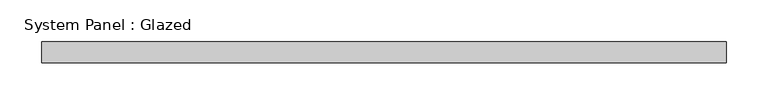
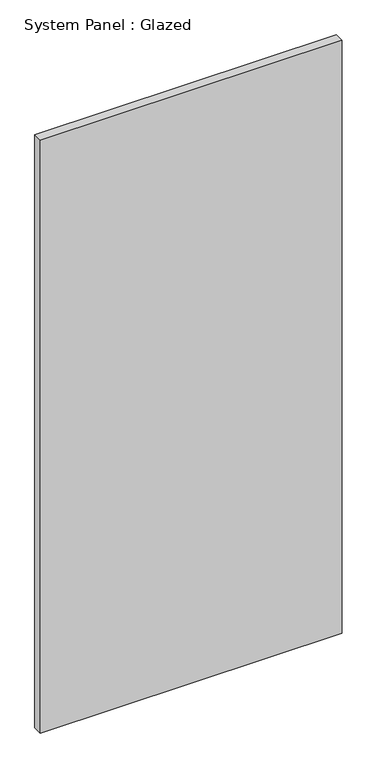
"""IFC4 building model written with IfcOpenShell, lengths in millimetres: plate geometry, System Panel : Glazed."""

from ifc_helpers import new_model, si_unit, origin, origin_with_axes, place, context, project, spatial, polyline, outline, extrude, source, transform, mapped, element, save


def system_panel_glazed_30879ba3(model_context):
    return source(origin(), model_context, "Body", "SweptSolid", [
        extrude(outline(polyline([(409.7761299, 19.05), (-409.7761299, 19.05), (-409.7761299, 44.45), (409.7761299, 44.45), (409.7761299, 19.05)])), origin_with_axes(), (0.0, 0.0, 1.0), 1701.8),
    ])


if __name__ == "__main__":
    model = new_model("IFC4")
    model_context = context("Model", 3, world=origin())
    ifc_project = project(units=[si_unit("LENGTHUNIT", "METRE", prefix="MILLI")], contexts=[model_context])
    site = spatial("IfcSite", under=ifc_project)
    building = spatial("IfcBuilding", under=site)
    placement = place(None, origin())
    system_panel_glazed_shape = system_panel_glazed_30879ba3(model_context)
    element("IfcPlate", 1, ObjectType="System Panel : Glazed", at=placement, inside=building, context=model_context, shape_type="MappedRepresentation", body=[
        mapped(system_panel_glazed_shape, transform((0.0, 0.0, 0.0), x_axis=(1.0, 0.0, 0.0), y_axis=(0.0, 1.0, 0.0), z_axis=(0.0, 0.0, 1.0))),
    ])
    save(model, "model.ifc")

# Revit data of these elements
# Type "System Panel : Glazed"
#   Construction Type Id = "GSP4R"
#   Analytic Construction = "1/8 in Pilkington single glazing"
#   Visual Light Transmittance = 0.9
#   Solar Heat Gain Coefficient = 0.86
#   Heat Transfer Coefficient (U) = 1.18115 BTU/(h·ft²·°F)
#   Define Thermal Properties by = 1
# Element 1 (IfcPlate, "System Panel : Glazed")
#   Materials on its faces: "Glass"
# Materials
#   "Glass": class "Glass", colour RGB 0 128 192, transparency 0.75, Description = "Soda Lime Glass", Cost = 0
